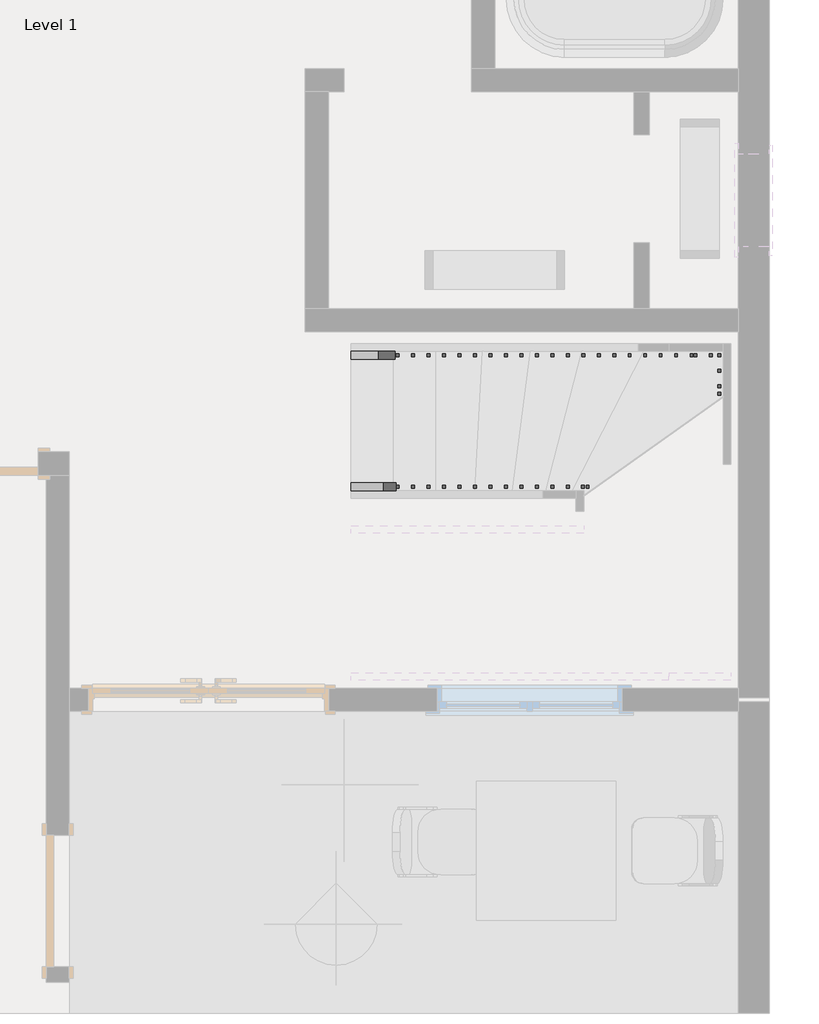
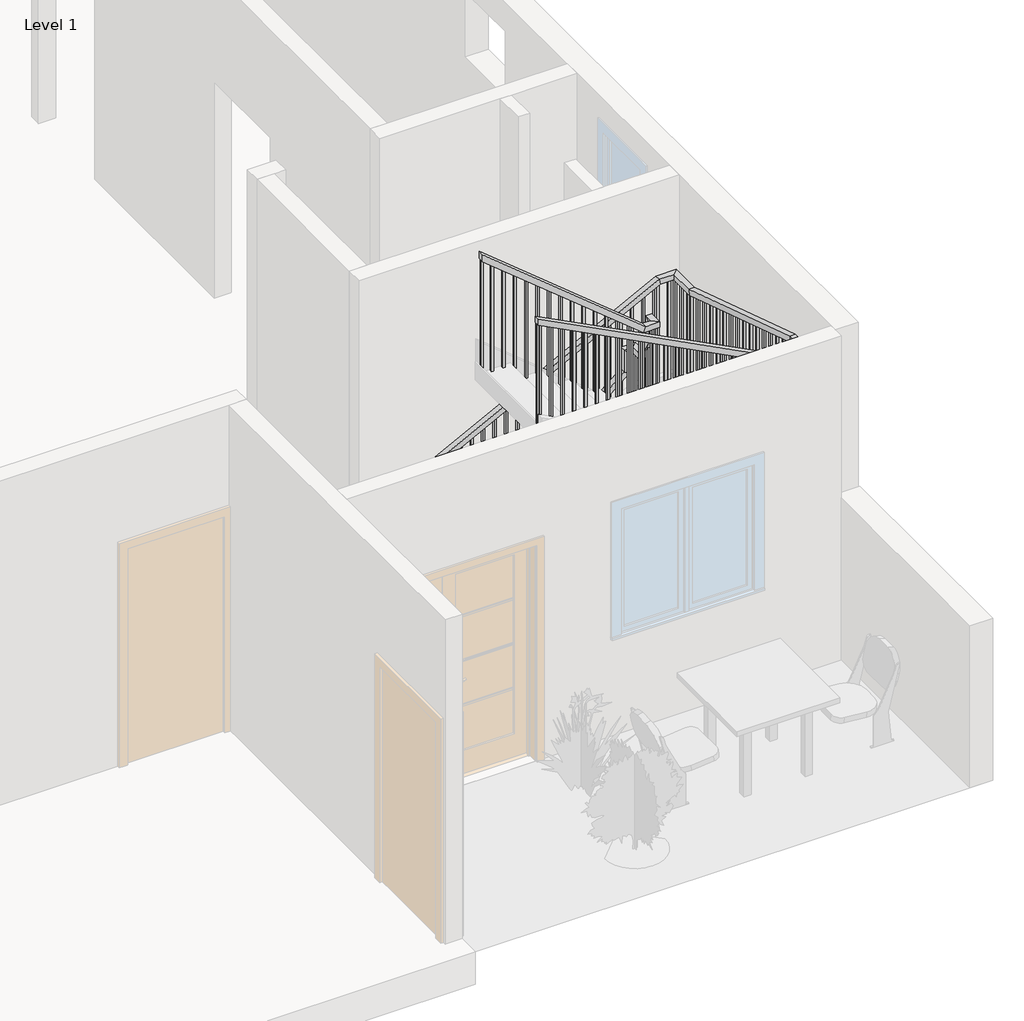
# One storey, part 2 of 3: 2 railings.
"""IFC4 building model written with IfcOpenShell, lengths in millimetres."""

from ifc_helpers import new_model, si_unit, frame, origin, place, context, project, spatial, polyline, outline, extrude, faceted_brep, element, save

model = new_model("IFC4")

# Units and contexts
model_context = context("Model", 3, world=origin())
ifc_project = project(units=[si_unit("LENGTHUNIT", "METRE", prefix="MILLI")], contexts=[model_context])

# Site, building, storey
site = spatial("IfcSite", under=ifc_project)
building = spatial("IfcBuilding", under=site)
storey = spatial("IfcBuildingStorey", under=building, Name="Level 1", Elevation=0.0)

# Railings
placement = place(None, origin())
element("IfcRailing", 1, ObjectType="Handrail - Rectangular", at=placement, inside=storey, context=model_context, shape_type="SolidModel", body=[
    faceted_brep([(-5644.7377406, -3148.8567046, 1025.2529681), (-5644.7377406, -3148.8567046, 959.7067088), (-5644.7377406, -3199.6567046, 959.7067088), (-5644.7377406, -3199.6567046, 1025.2529681), (-4193.2060487, -3148.8567046, 2208.7848338), (-4142.4060487, -3148.8567046, 2184.659247), (-4142.4060487, -3199.6567046, 2184.659247), (-4193.2060487, -3199.6567046, 2208.7848338), (-4193.2060487, -3148.8567046, 2414.6281882), (-4142.4060487, -3148.8567046, 2363.8281882), (-4142.4060487, -3199.6567046, 2363.8281882), (-4193.2060487, -3199.6567046, 2414.6281882), (-4066.2060487, -3148.8567046, 2414.6281882), (-4066.2060487, -3148.8567046, 2363.8281882), (-4117.0060487, -3199.6567046, 2363.8281882), (-4117.0060487, -3199.6567046, 2414.6281882), (-4066.2060487, -3275.8567046, 2414.6281882), (-4066.2060487, -3304.9780384, 2363.8281882), (-4117.0060487, -3304.9780384, 2363.8281882), (-4117.0060487, -3275.8567046, 2414.6281882), (-4066.2060487, -3402.8567046, 2631.5051451), (-4066.2060487, -3453.6567046, 2617.7256424), (-4117.0060487, -3453.6567046, 2617.7256424), (-4117.0060487, -3402.8567046, 2631.5051451), (-4066.2060487, -3402.8567046, 2837.3484995), (-4066.2060487, -3453.6567046, 2786.5484995), (-4117.0060487, -3453.6567046, 2786.5484995), (-4117.0060487, -3402.8567046, 2837.3484995), (-4066.2060487, -3529.8567046, 2837.3484995), (-4066.2060487, -3529.8567046, 2786.5484995), (-4117.0060487, -3479.0567046, 2786.5484995), (-4117.0060487, -3479.0567046, 2837.3484995), (-4193.2060487, -3529.8567046, 2837.3484995), (-4211.2914618, -3529.8567046, 2786.5484995), (-4211.2914618, -3479.0567046, 2786.5484995), (-4193.2060487, -3479.0567046, 2837.3484995), (-5644.7377406, -3529.8567046, 4020.8803652), (-5644.7377406, -3479.0567046, 4020.8803652), (-5644.7377406, -3479.0567046, 3955.3341059), (-5644.7377406, -3529.8567046, 3955.3341059)], [[[0, 1, 2, 3]], [[1, 0, 4, 5]], [[2, 1, 5, 6]], [[3, 2, 6, 7]], [[0, 3, 7, 4]], [[5, 4, 8, 9]], [[6, 5, 9, 10]], [[7, 6, 10, 11]], [[4, 7, 11, 8]], [[9, 8, 12, 13]], [[10, 9, 13, 14]], [[11, 10, 14, 15]], [[8, 11, 15, 12]], [[13, 12, 16, 17]], [[14, 13, 17, 18]], [[15, 14, 18, 19]], [[12, 15, 19, 16]], [[17, 16, 20, 21]], [[18, 17, 21, 22]], [[19, 18, 22, 23]], [[16, 19, 23, 20]], [[21, 20, 24, 25]], [[22, 21, 25, 26]], [[23, 22, 26, 27]], [[20, 23, 27, 24]], [[25, 24, 28, 29]], [[26, 25, 29, 30]], [[27, 26, 30, 31]], [[24, 27, 31, 28]], [[29, 28, 32, 33]], [[30, 29, 33, 34]], [[31, 30, 34, 35]], [[28, 31, 35, 32]], [[36, 37, 38, 39]], [[33, 32, 36, 39]], [[34, 33, 39, 38]], [[35, 34, 38, 37]], [[32, 35, 37, 36]]]),
    extrude(outline(polyline([(3866.2231262, -5535.4484051), (3881.7558784, -5554.4984051), (2878.6666667, -5554.4984051), (2878.6666667, -5535.4484051), (3866.2231262, -5535.4484051)])), frame((0.0, -3513.9817046, 0.0), z_axis=(0.0, 1.0, 0.0), x_axis=(0.0, 0.0, 1.0)), (0.0, 0.0, 1.0), 19.05),
    extrude(outline(polyline([(3783.3817813, -5433.8484051), (3798.9145334, -5452.8984051), (2878.6666667, -5452.8984051), (2878.6666667, -5433.8484051), (3783.3817813, -5433.8484051)])), frame((0.0, -3513.9817046, 0.0), z_axis=(0.0, 1.0, 0.0), x_axis=(0.0, 0.0, 1.0)), (0.0, 0.0, 1.0), 19.05),
    extrude(outline(polyline([(3700.5404364, -5332.2484051), (3716.0731885, -5351.2984051), (2709.3333333, -5351.2984051), (2709.3333333, -5332.2484051), (3700.5404364, -5332.2484051)])), frame((0.0, -3513.9817046, 0.0), z_axis=(0.0, 1.0, 0.0), x_axis=(0.0, 0.0, 1.0)), (0.0, 0.0, 1.0), 19.05),
    extrude(outline(polyline([(3617.6990914, -5230.6484051), (3633.2318436, -5249.6984051), (2709.3333333, -5249.6984051), (2709.3333333, -5230.6484051), (3617.6990914, -5230.6484051)])), frame((0.0, -3513.9817046, 0.0), z_axis=(0.0, 1.0, 0.0), x_axis=(0.0, 0.0, 1.0)), (0.0, 0.0, 1.0), 19.05),
    extrude(outline(polyline([(3534.8577465, -5129.0484051), (3550.3904987, -5148.0984051), (2709.3333333, -5148.0984051), (2709.3333333, -5129.0484051), (3534.8577465, -5129.0484051)])), frame((0.0, -3513.9817046, 0.0), z_axis=(0.0, 1.0, 0.0), x_axis=(0.0, 0.0, 1.0)), (0.0, 0.0, 1.0), 19.05),
    extrude(outline(polyline([(3452.0164016, -5027.4484051), (3467.5491538, -5046.4984051), (2540.0, -5046.4984051), (2540.0, -5027.4484051), (3452.0164016, -5027.4484051)])), frame((0.0, -3513.9817046, 0.0), z_axis=(0.0, 1.0, 0.0), x_axis=(0.0, 0.0, 1.0)), (0.0, 0.0, 1.0), 19.05),
    extrude(outline(polyline([(3369.1750567, -4925.8484051), (3384.7078088, -4944.8984051), (2540.0, -4944.8984051), (2540.0, -4925.8484051), (3369.1750567, -4925.8484051)])), frame((0.0, -3513.9817046, 0.0), z_axis=(0.0, 1.0, 0.0), x_axis=(0.0, 0.0, 1.0)), (0.0, 0.0, 1.0), 19.05),
    extrude(outline(polyline([(3286.3337117, -4824.2484051), (3301.8664639, -4843.2984051), (2540.0, -4843.2984051), (2540.0, -4824.2484051), (3286.3337117, -4824.2484051)])), frame((0.0, -3513.9817046, 0.0), z_axis=(0.0, 1.0, 0.0), x_axis=(0.0, 0.0, 1.0)), (0.0, 0.0, 1.0), 19.05),
    extrude(outline(polyline([(3203.4923668, -4722.6484051), (3219.025119, -4741.6984051), (2370.6666667, -4741.6984051), (2370.6666667, -4722.6484051), (3203.4923668, -4722.6484051)])), frame((0.0, -3513.9817046, 0.0), z_axis=(0.0, 1.0, 0.0), x_axis=(0.0, 0.0, 1.0)), (0.0, 0.0, 1.0), 19.05),
    extrude(outline(polyline([(3120.6510219, -4621.0484051), (3136.1837741, -4640.0984051), (2370.6666667, -4640.0984051), (2370.6666667, -4621.0484051), (3120.6510219, -4621.0484051)])), frame((0.0, -3513.9817046, 0.0), z_axis=(0.0, 1.0, 0.0), x_axis=(0.0, 0.0, 1.0)), (0.0, 0.0, 1.0), 19.05),
    extrude(outline(polyline([(3037.809677, -4519.4484051), (3053.3424291, -4538.4984051), (2201.3333333, -4538.4984051), (2201.3333333, -4519.4484051), (3037.809677, -4519.4484051)])), frame((0.0, -3513.9817046, 0.0), z_axis=(0.0, 1.0, 0.0), x_axis=(0.0, 0.0, 1.0)), (0.0, 0.0, 1.0), 19.05),
    extrude(outline(polyline([(2954.9683321, -4417.8484051), (2970.5010842, -4436.8984051), (2201.3333333, -4436.8984051), (2201.3333333, -4417.8484051), (2954.9683321, -4417.8484051)])), frame((0.0, -3513.9817046, 0.0), z_axis=(0.0, 1.0, 0.0), x_axis=(0.0, 0.0, 1.0)), (0.0, 0.0, 1.0), 19.05),
    extrude(outline(polyline([(2872.1269871, -4316.2484051), (2887.6597393, -4335.2984051), (2032.0, -4335.2984051), (2032.0, -4316.2484051), (2872.1269871, -4316.2484051)])), frame((0.0, -3513.9817046, 0.0), z_axis=(0.0, 1.0, 0.0), x_axis=(0.0, 0.0, 1.0)), (0.0, 0.0, 1.0), 19.05),
    extrude(outline(polyline([(2789.2856422, -4214.6484051), (2804.8183944, -4233.6984051), (2032.0, -4233.6984051), (2032.0, -4214.6484051), (2789.2856422, -4214.6484051)])), frame((0.0, -3513.9817046, 0.0), z_axis=(0.0, 1.0, 0.0), x_axis=(0.0, 0.0, 1.0)), (0.0, 0.0, 1.0), 19.05),
    extrude(outline(polyline([(-3401.7676083, 2529.115018), (-3382.7176083, 2496.5834745), (-3382.7176083, 1524.0), (-3401.7676083, 1524.0), (-3401.7676083, 2529.115018)])), frame((-4101.1310487, 0.0, 0.0), z_axis=(1.0, 0.0, 0.0), x_axis=(0.0, 1.0, 0.0)), (0.0, 0.0, 1.0), 19.05),
    extrude(outline(polyline([(-3300.1676083, 2355.6134525), (-3281.1176083, 2323.0819089), (-3281.1176083, 1524.0), (-3300.1676083, 1524.0), (-3300.1676083, 2355.6134525)])), frame((-4101.1310487, 0.0, 0.0), z_axis=(1.0, 0.0, 0.0), x_axis=(0.0, 1.0, 0.0)), (0.0, 0.0, 1.0), 19.05),
    extrude(outline(polyline([(2127.2519138, -4212.8127406), (2111.7191617, -4231.8627406), (1016.0, -4231.8627406), (1016.0, -4212.8127406), (2127.2519138, -4212.8127406)])), frame((0.0, -3183.7817046, 0.0), z_axis=(0.0, 1.0, 0.0), x_axis=(0.0, 0.0, 1.0)), (0.0, 0.0, 1.0), 19.05),
    extrude(outline(polyline([(2044.4105689, -4314.4127406), (2028.8778167, -4333.4627406), (1016.0, -4333.4627406), (1016.0, -4314.4127406), (2044.4105689, -4314.4127406)])), frame((0.0, -3183.7817046, 0.0), z_axis=(0.0, 1.0, 0.0), x_axis=(0.0, 0.0, 1.0)), (0.0, 0.0, 1.0), 19.05),
    extrude(outline(polyline([(1961.569224, -4416.0127406), (1946.0364718, -4435.0627406), (846.6666667, -4435.0627406), (846.6666667, -4416.0127406), (1961.569224, -4416.0127406)])), frame((0.0, -3183.7817046, 0.0), z_axis=(0.0, 1.0, 0.0), x_axis=(0.0, 0.0, 1.0)), (0.0, 0.0, 1.0), 19.05),
    extrude(outline(polyline([(1878.7278791, -4517.6127406), (1863.1951269, -4536.6627406), (846.6666667, -4536.6627406), (846.6666667, -4517.6127406), (1878.7278791, -4517.6127406)])), frame((0.0, -3183.7817046, 0.0), z_axis=(0.0, 1.0, 0.0), x_axis=(0.0, 0.0, 1.0)), (0.0, 0.0, 1.0), 19.05),
    extrude(outline(polyline([(1795.8865341, -4619.2127406), (1780.353782, -4638.2627406), (677.3333333, -4638.2627406), (677.3333333, -4619.2127406), (1795.8865341, -4619.2127406)])), frame((0.0, -3183.7817046, 0.0), z_axis=(0.0, 1.0, 0.0), x_axis=(0.0, 0.0, 1.0)), (0.0, 0.0, 1.0), 19.05),
    extrude(outline(polyline([(1713.0451892, -4720.8127406), (1697.5124371, -4739.8627406), (677.3333333, -4739.8627406), (677.3333333, -4720.8127406), (1713.0451892, -4720.8127406)])), frame((0.0, -3183.7817046, 0.0), z_axis=(0.0, 1.0, 0.0), x_axis=(0.0, 0.0, 1.0)), (0.0, 0.0, 1.0), 19.05),
    extrude(outline(polyline([(1630.2038443, -4822.4127406), (1614.6710921, -4841.4627406), (508.0, -4841.4627406), (508.0, -4822.4127406), (1630.2038443, -4822.4127406)])), frame((0.0, -3183.7817046, 0.0), z_axis=(0.0, 1.0, 0.0), x_axis=(0.0, 0.0, 1.0)), (0.0, 0.0, 1.0), 19.05),
    extrude(outline(polyline([(1547.3624994, -4924.0127406), (1531.8297472, -4943.0627406), (508.0, -4943.0627406), (508.0, -4924.0127406), (1547.3624994, -4924.0127406)])), frame((0.0, -3183.7817046, 0.0), z_axis=(0.0, 1.0, 0.0), x_axis=(0.0, 0.0, 1.0)), (0.0, 0.0, 1.0), 19.05),
    extrude(outline(polyline([(1464.5211545, -5025.6127406), (1448.9884023, -5044.6627406), (508.0, -5044.6627406), (508.0, -5025.6127406), (1464.5211545, -5025.6127406)])), frame((0.0, -3183.7817046, 0.0), z_axis=(0.0, 1.0, 0.0), x_axis=(0.0, 0.0, 1.0)), (0.0, 0.0, 1.0), 19.05),
    extrude(outline(polyline([(1381.6798095, -5127.2127406), (1366.1470574, -5146.2627406), (338.6666667, -5146.2627406), (338.6666667, -5127.2127406), (1381.6798095, -5127.2127406)])), frame((0.0, -3183.7817046, 0.0), z_axis=(0.0, 1.0, 0.0), x_axis=(0.0, 0.0, 1.0)), (0.0, 0.0, 1.0), 19.05),
    extrude(outline(polyline([(1298.8384646, -5228.8127406), (1283.3057124, -5247.8627406), (338.6666667, -5247.8627406), (338.6666667, -5228.8127406), (1298.8384646, -5228.8127406)])), frame((0.0, -3183.7817046, 0.0), z_axis=(0.0, 1.0, 0.0), x_axis=(0.0, 0.0, 1.0)), (0.0, 0.0, 1.0), 19.05),
    extrude(outline(polyline([(1215.9971197, -5330.4127406), (1200.4643675, -5349.4627406), (338.6666667, -5349.4627406), (338.6666667, -5330.4127406), (1215.9971197, -5330.4127406)])), frame((0.0, -3183.7817046, 0.0), z_axis=(0.0, 1.0, 0.0), x_axis=(0.0, 0.0, 1.0)), (0.0, 0.0, 1.0), 19.05),
    extrude(outline(polyline([(1133.1557748, -5432.0127406), (1117.6230226, -5451.0627406), (169.3333333, -5451.0627406), (169.3333333, -5432.0127406), (1133.1557748, -5432.0127406)])), frame((0.0, -3183.7817046, 0.0), z_axis=(0.0, 1.0, 0.0), x_axis=(0.0, 0.0, 1.0)), (0.0, 0.0, 1.0), 19.05),
    extrude(outline(polyline([(1050.3144298, -5533.6127406), (1034.7816777, -5552.6627406), (169.3333333, -5552.6627406), (169.3333333, -5533.6127406), (1050.3144298, -5533.6127406)])), frame((0.0, -3183.7817046, 0.0), z_axis=(0.0, 1.0, 0.0), x_axis=(0.0, 0.0, 1.0)), (0.0, 0.0, 1.0), 19.05),
    extrude(outline(polyline([(-4113.0484051, -3494.9317046), (-4113.0484051, -3513.9817046), (-4132.0984051, -3513.9817046), (-4132.0984051, -3494.9317046), (-4113.0484051, -3494.9317046)])), frame((0.0, 0.0, 1862.6666667), z_axis=(0.0, 0.0, 1.0), x_axis=(1.0, 0.0, 0.0)), (0.0, 0.0, 1.0), 923.8818329),
    extrude(outline(polyline([(-4101.1310487, -3494.9317046), (-4082.0810487, -3494.9317046), (-4082.0810487, -3513.9817046), (-4101.1310487, -3513.9817046), (-4101.1310487, -3494.9317046)])), frame((0.0, 0.0, 1862.6666667), z_axis=(0.0, 0.0, 1.0), x_axis=(1.0, 0.0, 0.0)), (0.0, 0.0, 1.0), 923.8818329),
    extrude(outline(polyline([(-4101.1310487, -3480.1458008), (-4082.0810487, -3480.1458008), (-4082.0810487, -3499.1958008), (-4101.1310487, -3499.1958008), (-4101.1310487, -3480.1458008)])), frame((0.0, 0.0, 1693.3333333), z_axis=(0.0, 0.0, 1.0), x_axis=(1.0, 0.0, 0.0)), (0.0, 0.0, 1.0), 1093.2151662),
    extrude(outline(polyline([(-4101.1310487, -3179.5176083), (-4082.0810487, -3179.5176083), (-4082.0810487, -3198.5676083), (-4101.1310487, -3198.5676083), (-4101.1310487, -3179.5176083)])), frame((0.0, 0.0, 1354.6666667), z_axis=(0.0, 0.0, 1.0), x_axis=(1.0, 0.0, 0.0)), (0.0, 0.0, 1.0), 1009.1615215),
    extrude(outline(polyline([(-4101.1310487, -3183.7817046), (-4101.1310487, -3164.7317046), (-4082.0810487, -3164.7317046), (-4082.0810487, -3183.7817046), (-4101.1310487, -3183.7817046)])), frame((0.0, 0.0, 1185.3333333), z_axis=(0.0, 0.0, 1.0), x_axis=(1.0, 0.0, 0.0)), (0.0, 0.0, 1.0), 1178.4948549),
    extrude(outline(polyline([(-4132.0984051, -3183.7817046), (-4132.0984051, -3164.7317046), (-4113.0484051, -3164.7317046), (-4113.0484051, -3183.7817046), (-4132.0984051, -3183.7817046)])), frame((0.0, 0.0, 1185.3333333), z_axis=(0.0, 0.0, 1.0), x_axis=(1.0, 0.0, 0.0)), (0.0, 0.0, 1.0), 1178.4948549),
    extrude(outline(polyline([(3939.8013537, -5625.6877406), (3955.3341059, -5644.7377406), (2878.6666667, -5644.7377406), (2878.6666667, -5625.6877406), (3939.8013537, -5625.6877406)])), frame((0.0, -3513.9817046, 0.0), z_axis=(0.0, 1.0, 0.0), x_axis=(0.0, 0.0, 1.0)), (0.0, 0.0, 1.0), 19.05),
    extrude(outline(polyline([(975.239461, -5625.6877406), (959.7067088, -5644.7377406), (169.3333333, -5644.7377406), (169.3333333, -5625.6877406), (975.239461, -5625.6877406)])), frame((0.0, -3183.7817046, 0.0), z_axis=(0.0, 1.0, 0.0), x_axis=(0.0, 0.0, 1.0)), (0.0, 0.0, 1.0), 19.05),
])
element("IfcRailing", 2, ObjectType="Handrail - Rectangular", at=placement, inside=storey, context=model_context, shape_type="SolidModel", body=[
    faceted_brep([(-5644.7377406, -2285.2567046, 1109.0771751), (-5644.7377406, -2285.2567046, 1051.9280057), (-5644.7377406, -2336.0567046, 1051.9280057), (-5644.7377406, -2336.0567046, 1109.0771751), (-3384.7558841, -2285.2567046, 2273.7644996), (-3372.4358328, -2285.2567046, 2222.9644996), (-3372.4358328, -2336.0567046, 2222.9644996), (-3384.7558841, -2336.0567046, 2273.7644996), (-3202.6060487, -2285.2567046, 2273.7644996), (-3202.6060487, -2285.2567046, 2222.9644996), (-3253.4060487, -2336.0567046, 2222.9644996), (-3253.4060487, -2336.0567046, 2273.7644996), (-3202.6060487, -2562.4106572, 2273.7644996), (-3202.6060487, -2570.3612333, 2222.9644996), (-3253.4060487, -2570.3612333, 2222.9644996), (-3253.4060487, -2562.4106572, 2273.7644996), (-3202.6060487, -4116.3027519, 2772.3688337), (-3202.6060487, -4124.2533281, 2721.5688337), (-3253.4060487, -4124.2533281, 2721.5688337), (-3253.4060487, -4116.3027519, 2772.3688337), (-3202.6060487, -4393.4567046, 2772.3688337), (-3202.6060487, -4393.4567046, 2721.5688337), (-3253.4060487, -4342.6567046, 2721.5688337), (-3253.4060487, -4342.6567046, 2772.3688337), (-3384.7558841, -4393.4567046, 2772.3688337), (-3397.0759354, -4393.4567046, 2721.5688337), (-3397.0759354, -4342.6567046, 2721.5688337), (-3384.7558841, -4342.6567046, 2772.3688337), (-5644.7377406, -4393.4567046, 3937.0561582), (-5644.7377406, -4342.6567046, 3937.0561582), (-5644.7377406, -4342.6567046, 3879.9069889), (-5644.7377406, -4393.4567046, 3879.9069889)], [[[0, 1, 2, 3]], [[1, 0, 4, 5]], [[2, 1, 5, 6]], [[3, 2, 6, 7]], [[0, 3, 7, 4]], [[5, 4, 8, 9]], [[6, 5, 9, 10]], [[7, 6, 10, 11]], [[4, 7, 11, 8]], [[9, 8, 12, 13]], [[10, 9, 13, 14]], [[11, 10, 14, 15]], [[8, 11, 15, 12]], [[13, 12, 16, 17]], [[14, 13, 17, 18]], [[15, 14, 18, 19]], [[12, 15, 19, 16]], [[17, 16, 20, 21]], [[18, 17, 21, 22]], [[19, 18, 22, 23]], [[16, 19, 23, 20]], [[21, 20, 24, 25]], [[22, 21, 25, 26]], [[23, 22, 26, 27]], [[20, 23, 27, 24]], [[28, 29, 30, 31]], [[25, 24, 28, 31]], [[26, 25, 31, 30]], [[27, 26, 30, 29]], [[24, 27, 29, 28]]]),
    extrude(outline(polyline([(3872.0443296, -5629.4808841), (2878.6666667, -5629.4808841), (2878.6666667, -5610.4308841), (3862.2268642, -5610.4308841), (3872.0443296, -5629.4808841)])), frame((0.0, -4377.5817046, 0.0), z_axis=(0.0, 1.0, 0.0), x_axis=(0.0, 0.0, 1.0)), (0.0, 0.0, 1.0), 19.05),
    extrude(outline(polyline([(3819.6845145, -5527.8808841), (2878.6666667, -5527.8808841), (2878.6666667, -5508.8308841), (3809.8670491, -5508.8308841), (3819.6845145, -5527.8808841)])), frame((0.0, -4377.5817046, 0.0), z_axis=(0.0, 1.0, 0.0), x_axis=(0.0, 0.0, 1.0)), (0.0, 0.0, 1.0), 19.05),
    extrude(outline(polyline([(3767.3246993, -5426.2808841), (2878.6666667, -5426.2808841), (2878.6666667, -5407.2308841), (3757.507234, -5407.2308841), (3767.3246993, -5426.2808841)])), frame((0.0, -4377.5817046, 0.0), z_axis=(0.0, 1.0, 0.0), x_axis=(0.0, 0.0, 1.0)), (0.0, 0.0, 1.0), 19.05),
    extrude(outline(polyline([(3714.9648842, -5324.6808841), (2709.3333333, -5324.6808841), (2709.3333333, -5305.6308841), (3705.1474189, -5305.6308841), (3714.9648842, -5324.6808841)])), frame((0.0, -4377.5817046, 0.0), z_axis=(0.0, 1.0, 0.0), x_axis=(0.0, 0.0, 1.0)), (0.0, 0.0, 1.0), 19.05),
    extrude(outline(polyline([(3662.6050691, -5223.0808841), (2709.3333333, -5223.0808841), (2709.3333333, -5204.0308841), (3652.7876038, -5204.0308841), (3662.6050691, -5223.0808841)])), frame((0.0, -4377.5817046, 0.0), z_axis=(0.0, 1.0, 0.0), x_axis=(0.0, 0.0, 1.0)), (0.0, 0.0, 1.0), 19.05),
    extrude(outline(polyline([(3610.245254, -5121.4808841), (2709.3333333, -5121.4808841), (2709.3333333, -5102.4308841), (3600.4277887, -5102.4308841), (3610.245254, -5121.4808841)])), frame((0.0, -4377.5817046, 0.0), z_axis=(0.0, 1.0, 0.0), x_axis=(0.0, 0.0, 1.0)), (0.0, 0.0, 1.0), 19.05),
    extrude(outline(polyline([(3557.8854389, -5019.8808841), (2540.0, -5019.8808841), (2540.0, -5000.8308841), (3548.0679735, -5000.8308841), (3557.8854389, -5019.8808841)])), frame((0.0, -4377.5817046, 0.0), z_axis=(0.0, 1.0, 0.0), x_axis=(0.0, 0.0, 1.0)), (0.0, 0.0, 1.0), 19.05),
    extrude(outline(polyline([(3505.5256238, -4918.2808841), (2540.0, -4918.2808841), (2540.0, -4899.2308841), (3495.7081584, -4899.2308841), (3505.5256238, -4918.2808841)])), frame((0.0, -4377.5817046, 0.0), z_axis=(0.0, 1.0, 0.0), x_axis=(0.0, 0.0, 1.0)), (0.0, 0.0, 1.0), 19.05),
    extrude(outline(polyline([(3453.1658086, -4816.6808841), (2540.0, -4816.6808841), (2540.0, -4797.6308841), (3443.3483433, -4797.6308841), (3453.1658086, -4816.6808841)])), frame((0.0, -4377.5817046, 0.0), z_axis=(0.0, 1.0, 0.0), x_axis=(0.0, 0.0, 1.0)), (0.0, 0.0, 1.0), 19.05),
    extrude(outline(polyline([(3400.8059935, -4715.0808841), (2370.6666667, -4715.0808841), (2370.6666667, -4696.0308841), (3390.9885282, -4696.0308841), (3400.8059935, -4715.0808841)])), frame((0.0, -4377.5817046, 0.0), z_axis=(0.0, 1.0, 0.0), x_axis=(0.0, 0.0, 1.0)), (0.0, 0.0, 1.0), 19.05),
    extrude(outline(polyline([(3348.4461784, -4613.4808841), (2370.6666667, -4613.4808841), (2370.6666667, -4594.4308841), (3338.6287131, -4594.4308841), (3348.4461784, -4613.4808841)])), frame((0.0, -4377.5817046, 0.0), z_axis=(0.0, 1.0, 0.0), x_axis=(0.0, 0.0, 1.0)), (0.0, 0.0, 1.0), 19.05),
    extrude(outline(polyline([(3296.0863633, -4511.8808841), (2370.6666667, -4511.8808841), (2370.6666667, -4492.8308841), (3286.268898, -4492.8308841), (3296.0863633, -4511.8808841)])), frame((0.0, -4377.5817046, 0.0), z_axis=(0.0, 1.0, 0.0), x_axis=(0.0, 0.0, 1.0)), (0.0, 0.0, 1.0), 19.05),
    extrude(outline(polyline([(3243.7265482, -4410.2808841), (2201.3333333, -4410.2808841), (2201.3333333, -4391.2308841), (3233.9090828, -4391.2308841), (3243.7265482, -4410.2808841)])), frame((0.0, -4377.5817046, 0.0), z_axis=(0.0, 1.0, 0.0), x_axis=(0.0, 0.0, 1.0)), (0.0, 0.0, 1.0), 19.05),
    extrude(outline(polyline([(3191.3667331, -4308.6808841), (2201.3333333, -4308.6808841), (2201.3333333, -4289.6308841), (3181.5492677, -4289.6308841), (3191.3667331, -4308.6808841)])), frame((0.0, -4377.5817046, 0.0), z_axis=(0.0, 1.0, 0.0), x_axis=(0.0, 0.0, 1.0)), (0.0, 0.0, 1.0), 19.05),
    extrude(outline(polyline([(3139.0069179, -4207.0808841), (2201.3333333, -4207.0808841), (2201.3333333, -4188.0308841), (3129.1894526, -4188.0308841), (3139.0069179, -4207.0808841)])), frame((0.0, -4377.5817046, 0.0), z_axis=(0.0, 1.0, 0.0), x_axis=(0.0, 0.0, 1.0)), (0.0, 0.0, 1.0), 19.05),
    extrude(outline(polyline([(3086.6471028, -4105.4808841), (2032.0, -4105.4808841), (2032.0, -4086.4308841), (3076.8296375, -4086.4308841), (3086.6471028, -4105.4808841)])), frame((0.0, -4377.5817046, 0.0), z_axis=(0.0, 1.0, 0.0), x_axis=(0.0, 0.0, 1.0)), (0.0, 0.0, 1.0), 19.05),
    extrude(outline(polyline([(3034.2872877, -4003.8808841), (2032.0, -4003.8808841), (2032.0, -3984.8308841), (3024.4698224, -3984.8308841), (3034.2872877, -4003.8808841)])), frame((0.0, -4377.5817046, 0.0), z_axis=(0.0, 1.0, 0.0), x_axis=(0.0, 0.0, 1.0)), (0.0, 0.0, 1.0), 19.05),
    extrude(outline(polyline([(2981.9274726, -3902.2808841), (2032.0, -3902.2808841), (2032.0, -3883.2308841), (2972.1100073, -3883.2308841), (2981.9274726, -3902.2808841)])), frame((0.0, -4377.5817046, 0.0), z_axis=(0.0, 1.0, 0.0), x_axis=(0.0, 0.0, 1.0)), (0.0, 0.0, 1.0), 19.05),
    extrude(outline(polyline([(2929.5676575, -3800.6808841), (2032.0, -3800.6808841), (2032.0, -3781.6308841), (2919.7501921, -3781.6308841), (2929.5676575, -3800.6808841)])), frame((0.0, -4377.5817046, 0.0), z_axis=(0.0, 1.0, 0.0), x_axis=(0.0, 0.0, 1.0)), (0.0, 0.0, 1.0), 19.05),
    extrude(outline(polyline([(2877.2078424, -3699.0808841), (1862.6666667, -3699.0808841), (1862.6666667, -3680.0308841), (2867.390377, -3680.0308841), (2877.2078424, -3699.0808841)])), frame((0.0, -4377.5817046, 0.0), z_axis=(0.0, 1.0, 0.0), x_axis=(0.0, 0.0, 1.0)), (0.0, 0.0, 1.0), 19.05),
    extrude(outline(polyline([(2824.8480272, -3597.4808841), (1862.6666667, -3597.4808841), (1862.6666667, -3578.4308841), (2815.0305619, -3578.4308841), (2824.8480272, -3597.4808841)])), frame((0.0, -4377.5817046, 0.0), z_axis=(0.0, 1.0, 0.0), x_axis=(0.0, 0.0, 1.0)), (0.0, 0.0, 1.0), 19.05),
    extrude(outline(polyline([(2772.4882121, -3495.8808841), (1862.6666667, -3495.8808841), (1862.6666667, -3476.8308841), (2762.6707468, -3476.8308841), (2772.4882121, -3495.8808841)])), frame((0.0, -4377.5817046, 0.0), z_axis=(0.0, 1.0, 0.0), x_axis=(0.0, 0.0, 1.0)), (0.0, 0.0, 1.0), 19.05),
    extrude(outline(polyline([(-3320.0810487, -4377.5817046), (-3339.1310487, -4377.5817046), (-3339.1310487, -4358.5317046), (-3320.0810487, -4358.5317046), (-3320.0810487, -4377.5817046)])), frame((0.0, 0.0, 1862.6666667), z_axis=(0.0, 0.0, 1.0), x_axis=(1.0, 0.0, 0.0)), (0.0, 0.0, 1.0), 858.902167),
    extrude(outline(polyline([(-3218.4810487, -4309.9777519), (-3218.4810487, -4329.0277519), (-3237.5310487, -4329.0277519), (-3237.5310487, -4309.9777519), (-3218.4810487, -4309.9777519)])), frame((0.0, 0.0, 1862.6666667), z_axis=(0.0, 0.0, 1.0), x_axis=(1.0, 0.0, 0.0)), (0.0, 0.0, 1.0), 858.902167),
    extrude(outline(polyline([(-3218.4810487, -4208.3777519), (-3218.4810487, -4227.4277519), (-3237.5310487, -4227.4277519), (-3237.5310487, -4208.3777519), (-3218.4810487, -4208.3777519)])), frame((0.0, 0.0, 1862.6666667), z_axis=(0.0, 0.0, 1.0), x_axis=(1.0, 0.0, 0.0)), (0.0, 0.0, 1.0), 858.902167),
    extrude(outline(polyline([(-4076.8856572, 2706.3697564), (-4076.8856572, 1693.3333333), (-4095.9356572, 1693.3333333), (-4095.9356572, 2712.4824155), (-4076.8856572, 2706.3697564)])), frame((-3237.5310487, 0.0, 0.0), z_axis=(1.0, 0.0, 0.0), x_axis=(0.0, 1.0, 0.0)), (0.0, 0.0, 1.0), 19.05),
    extrude(outline(polyline([(-3975.2856572, 2673.7689082), (-3975.2856572, 1693.3333333), (-3994.3356572, 1693.3333333), (-3994.3356572, 2679.8815673), (-3975.2856572, 2673.7689082)])), frame((-3237.5310487, 0.0, 0.0), z_axis=(1.0, 0.0, 0.0), x_axis=(0.0, 1.0, 0.0)), (0.0, 0.0, 1.0), 19.05),
    extrude(outline(polyline([(-3873.6856572, 2641.16806), (-3873.6856572, 1693.3333333), (-3892.7356572, 1693.3333333), (-3892.7356572, 2647.280719), (-3873.6856572, 2641.16806)])), frame((-3237.5310487, 0.0, 0.0), z_axis=(1.0, 0.0, 0.0), x_axis=(0.0, 1.0, 0.0)), (0.0, 0.0, 1.0), 19.05),
    extrude(outline(polyline([(-3772.0856572, 2608.5672118), (-3772.0856572, 1693.3333333), (-3791.1356572, 1693.3333333), (-3791.1356572, 2614.6798708), (-3772.0856572, 2608.5672118)])), frame((-3237.5310487, 0.0, 0.0), z_axis=(1.0, 0.0, 0.0), x_axis=(0.0, 1.0, 0.0)), (0.0, 0.0, 1.0), 19.05),
    extrude(outline(polyline([(-3670.4856572, 2575.9663635), (-3670.4856572, 1693.3333333), (-3689.5356572, 1693.3333333), (-3689.5356572, 2582.0790226), (-3670.4856572, 2575.9663635)])), frame((-3237.5310487, 0.0, 0.0), z_axis=(1.0, 0.0, 0.0), x_axis=(0.0, 1.0, 0.0)), (0.0, 0.0, 1.0), 19.05),
    extrude(outline(polyline([(-3568.8856572, 2543.3655153), (-3568.8856572, 1693.3333333), (-3587.9356572, 1693.3333333), (-3587.9356572, 2549.4781744), (-3568.8856572, 2543.3655153)])), frame((-3237.5310487, 0.0, 0.0), z_axis=(1.0, 0.0, 0.0), x_axis=(0.0, 1.0, 0.0)), (0.0, 0.0, 1.0), 19.05),
    extrude(outline(polyline([(-3467.2856572, 2510.7646671), (-3467.2856572, 1524.0), (-3486.3356572, 1524.0), (-3486.3356572, 2516.8773261), (-3467.2856572, 2510.7646671)])), frame((-3237.5310487, 0.0, 0.0), z_axis=(1.0, 0.0, 0.0), x_axis=(0.0, 1.0, 0.0)), (0.0, 0.0, 1.0), 19.05),
    extrude(outline(polyline([(-3365.6856572, 2478.1638189), (-3365.6856572, 1524.0), (-3384.7356572, 1524.0), (-3384.7356572, 2484.2764779), (-3365.6856572, 2478.1638189)])), frame((-3237.5310487, 0.0, 0.0), z_axis=(1.0, 0.0, 0.0), x_axis=(0.0, 1.0, 0.0)), (0.0, 0.0, 1.0), 19.05),
    extrude(outline(polyline([(-3264.0856572, 2445.5629706), (-3264.0856572, 1524.0), (-3283.1356572, 1524.0), (-3283.1356572, 2451.6756297), (-3264.0856572, 2445.5629706)])), frame((-3237.5310487, 0.0, 0.0), z_axis=(1.0, 0.0, 0.0), x_axis=(0.0, 1.0, 0.0)), (0.0, 0.0, 1.0), 19.05),
    extrude(outline(polyline([(-3162.4856572, 2412.9621224), (-3162.4856572, 1524.0), (-3181.5356572, 1524.0), (-3181.5356572, 2419.0747814), (-3162.4856572, 2412.9621224)])), frame((-3237.5310487, 0.0, 0.0), z_axis=(1.0, 0.0, 0.0), x_axis=(0.0, 1.0, 0.0)), (0.0, 0.0, 1.0), 19.05),
    extrude(outline(polyline([(-3060.8856572, 2380.3612742), (-3060.8856572, 1354.6666667), (-3079.9356572, 1354.6666667), (-3079.9356572, 2386.4739332), (-3060.8856572, 2380.3612742)])), frame((-3237.5310487, 0.0, 0.0), z_axis=(1.0, 0.0, 0.0), x_axis=(0.0, 1.0, 0.0)), (0.0, 0.0, 1.0), 19.05),
    extrude(outline(polyline([(-2959.2856572, 2347.7604259), (-2959.2856572, 1354.6666667), (-2978.3356572, 1354.6666667), (-2978.3356572, 2353.873085), (-2959.2856572, 2347.7604259)])), frame((-3237.5310487, 0.0, 0.0), z_axis=(1.0, 0.0, 0.0), x_axis=(0.0, 1.0, 0.0)), (0.0, 0.0, 1.0), 19.05),
    extrude(outline(polyline([(-2857.6856572, 2315.1595777), (-2857.6856572, 1354.6666667), (-2876.7356572, 1354.6666667), (-2876.7356572, 2321.2722368), (-2857.6856572, 2315.1595777)])), frame((-3237.5310487, 0.0, 0.0), z_axis=(1.0, 0.0, 0.0), x_axis=(0.0, 1.0, 0.0)), (0.0, 0.0, 1.0), 19.05),
    extrude(outline(polyline([(-2756.0856572, 2282.5587295), (-2756.0856572, 1354.6666667), (-2775.1356572, 1354.6666667), (-2775.1356572, 2288.6713885), (-2756.0856572, 2282.5587295)])), frame((-3237.5310487, 0.0, 0.0), z_axis=(1.0, 0.0, 0.0), x_axis=(0.0, 1.0, 0.0)), (0.0, 0.0, 1.0), 19.05),
    extrude(outline(polyline([(-2654.4856572, 2249.9578813), (-2654.4856572, 1354.6666667), (-2673.5356572, 1354.6666667), (-2673.5356572, 2256.0705403), (-2654.4856572, 2249.9578813)])), frame((-3237.5310487, 0.0, 0.0), z_axis=(1.0, 0.0, 0.0), x_axis=(0.0, 1.0, 0.0)), (0.0, 0.0, 1.0), 19.05),
    extrude(outline(polyline([(-3218.4810487, -2504.3317046), (-3218.4810487, -2523.3817046), (-3237.5310487, -2523.3817046), (-3237.5310487, -2504.3317046), (-3218.4810487, -2504.3317046)])), frame((0.0, 0.0, 1185.3333333), z_axis=(0.0, 0.0, 1.0), x_axis=(1.0, 0.0, 0.0)), (0.0, 0.0, 1.0), 1037.6311663),
    extrude(outline(polyline([(-3218.4810487, -2402.7317046), (-3218.4810487, -2421.7817046), (-3237.5310487, -2421.7817046), (-3237.5310487, -2402.7317046), (-3218.4810487, -2402.7317046)])), frame((0.0, 0.0, 1185.3333333), z_axis=(0.0, 0.0, 1.0), x_axis=(1.0, 0.0, 0.0)), (0.0, 0.0, 1.0), 1037.6311663),
    extrude(outline(polyline([(-3292.6808841, -2301.1317046), (-3273.6308841, -2301.1317046), (-3273.6308841, -2320.1817046), (-3292.6808841, -2320.1817046), (-3292.6808841, -2301.1317046)])), frame((0.0, 0.0, 1185.3333333), z_axis=(0.0, 0.0, 1.0), x_axis=(1.0, 0.0, 0.0)), (0.0, 0.0, 1.0), 1037.6311663),
    extrude(outline(polyline([(2198.9352056, -3419.0627406), (1185.3333333, -3419.0627406), (1185.3333333, -3400.0127406), (2208.752671, -3400.0127406), (2198.9352056, -3419.0627406)])), frame((0.0, -2320.1817046, 0.0), z_axis=(0.0, 1.0, 0.0), x_axis=(0.0, 0.0, 1.0)), (0.0, 0.0, 1.0), 19.05),
    extrude(outline(polyline([(2146.5753905, -3520.6627406), (1185.3333333, -3520.6627406), (1185.3333333, -3501.6127406), (2156.3928558, -3501.6127406), (2146.5753905, -3520.6627406)])), frame((0.0, -2320.1817046, 0.0), z_axis=(0.0, 1.0, 0.0), x_axis=(0.0, 0.0, 1.0)), (0.0, 0.0, 1.0), 19.05),
    extrude(outline(polyline([(2094.2155754, -3622.2627406), (1185.3333333, -3622.2627406), (1185.3333333, -3603.2127406), (2104.0330407, -3603.2127406), (2094.2155754, -3622.2627406)])), frame((0.0, -2320.1817046, 0.0), z_axis=(0.0, 1.0, 0.0), x_axis=(0.0, 0.0, 1.0)), (0.0, 0.0, 1.0), 19.05),
    extrude(outline(polyline([(2041.8557603, -3723.8627406), (1185.3333333, -3723.8627406), (1185.3333333, -3704.8127406), (2051.6732256, -3704.8127406), (2041.8557603, -3723.8627406)])), frame((0.0, -2320.1817046, 0.0), z_axis=(0.0, 1.0, 0.0), x_axis=(0.0, 0.0, 1.0)), (0.0, 0.0, 1.0), 19.05),
    extrude(outline(polyline([(1989.4959452, -3825.4627406), (1016.0, -3825.4627406), (1016.0, -3806.4127406), (1999.3134105, -3806.4127406), (1989.4959452, -3825.4627406)])), frame((0.0, -2320.1817046, 0.0), z_axis=(0.0, 1.0, 0.0), x_axis=(0.0, 0.0, 1.0)), (0.0, 0.0, 1.0), 19.05),
    extrude(outline(polyline([(1937.13613, -3927.0627406), (1016.0, -3927.0627406), (1016.0, -3908.0127406), (1946.9535954, -3908.0127406), (1937.13613, -3927.0627406)])), frame((0.0, -2320.1817046, 0.0), z_axis=(0.0, 1.0, 0.0), x_axis=(0.0, 0.0, 1.0)), (0.0, 0.0, 1.0), 19.05),
    extrude(outline(polyline([(1884.7763149, -4028.6627406), (1016.0, -4028.6627406), (1016.0, -4009.6127406), (1894.5937803, -4009.6127406), (1884.7763149, -4028.6627406)])), frame((0.0, -2320.1817046, 0.0), z_axis=(0.0, 1.0, 0.0), x_axis=(0.0, 0.0, 1.0)), (0.0, 0.0, 1.0), 19.05),
    extrude(outline(polyline([(1832.4164998, -4130.2627406), (1016.0, -4130.2627406), (1016.0, -4111.2127406), (1842.2339651, -4111.2127406), (1832.4164998, -4130.2627406)])), frame((0.0, -2320.1817046, 0.0), z_axis=(0.0, 1.0, 0.0), x_axis=(0.0, 0.0, 1.0)), (0.0, 0.0, 1.0), 19.05),
    extrude(outline(polyline([(1780.0566847, -4231.8627406), (846.6666667, -4231.8627406), (846.6666667, -4212.8127406), (1789.87415, -4212.8127406), (1780.0566847, -4231.8627406)])), frame((0.0, -2320.1817046, 0.0), z_axis=(0.0, 1.0, 0.0), x_axis=(0.0, 0.0, 1.0)), (0.0, 0.0, 1.0), 19.05),
    extrude(outline(polyline([(1727.6968696, -4333.4627406), (846.6666667, -4333.4627406), (846.6666667, -4314.4127406), (1737.5143349, -4314.4127406), (1727.6968696, -4333.4627406)])), frame((0.0, -2320.1817046, 0.0), z_axis=(0.0, 1.0, 0.0), x_axis=(0.0, 0.0, 1.0)), (0.0, 0.0, 1.0), 19.05),
    extrude(outline(polyline([(1675.3370545, -4435.0627406), (846.6666667, -4435.0627406), (846.6666667, -4416.0127406), (1685.1545198, -4416.0127406), (1675.3370545, -4435.0627406)])), frame((0.0, -2320.1817046, 0.0), z_axis=(0.0, 1.0, 0.0), x_axis=(0.0, 0.0, 1.0)), (0.0, 0.0, 1.0), 19.05),
    extrude(outline(polyline([(1622.9772393, -4536.6627406), (677.3333333, -4536.6627406), (677.3333333, -4517.6127406), (1632.7947047, -4517.6127406), (1622.9772393, -4536.6627406)])), frame((0.0, -2320.1817046, 0.0), z_axis=(0.0, 1.0, 0.0), x_axis=(0.0, 0.0, 1.0)), (0.0, 0.0, 1.0), 19.05),
    extrude(outline(polyline([(1570.6174242, -4638.2627406), (677.3333333, -4638.2627406), (677.3333333, -4619.2127406), (1580.4348896, -4619.2127406), (1570.6174242, -4638.2627406)])), frame((0.0, -2320.1817046, 0.0), z_axis=(0.0, 1.0, 0.0), x_axis=(0.0, 0.0, 1.0)), (0.0, 0.0, 1.0), 19.05),
    extrude(outline(polyline([(1518.2576091, -4739.8627406), (677.3333333, -4739.8627406), (677.3333333, -4720.8127406), (1528.0750744, -4720.8127406), (1518.2576091, -4739.8627406)])), frame((0.0, -2320.1817046, 0.0), z_axis=(0.0, 1.0, 0.0), x_axis=(0.0, 0.0, 1.0)), (0.0, 0.0, 1.0), 19.05),
    extrude(outline(polyline([(1465.897794, -4841.4627406), (508.0, -4841.4627406), (508.0, -4822.4127406), (1475.7152593, -4822.4127406), (1465.897794, -4841.4627406)])), frame((0.0, -2320.1817046, 0.0), z_axis=(0.0, 1.0, 0.0), x_axis=(0.0, 0.0, 1.0)), (0.0, 0.0, 1.0), 19.05),
    extrude(outline(polyline([(1413.5379789, -4943.0627406), (508.0, -4943.0627406), (508.0, -4924.0127406), (1423.3554442, -4924.0127406), (1413.5379789, -4943.0627406)])), frame((0.0, -2320.1817046, 0.0), z_axis=(0.0, 1.0, 0.0), x_axis=(0.0, 0.0, 1.0)), (0.0, 0.0, 1.0), 19.05),
    extrude(outline(polyline([(1361.1781638, -5044.6627406), (508.0, -5044.6627406), (508.0, -5025.6127406), (1370.9956291, -5025.6127406), (1361.1781638, -5044.6627406)])), frame((0.0, -2320.1817046, 0.0), z_axis=(0.0, 1.0, 0.0), x_axis=(0.0, 0.0, 1.0)), (0.0, 0.0, 1.0), 19.05),
    extrude(outline(polyline([(1308.8183486, -5146.2627406), (338.6666667, -5146.2627406), (338.6666667, -5127.2127406), (1318.635814, -5127.2127406), (1308.8183486, -5146.2627406)])), frame((0.0, -2320.1817046, 0.0), z_axis=(0.0, 1.0, 0.0), x_axis=(0.0, 0.0, 1.0)), (0.0, 0.0, 1.0), 19.05),
    extrude(outline(polyline([(1256.4585335, -5247.8627406), (338.6666667, -5247.8627406), (338.6666667, -5228.8127406), (1266.2759989, -5228.8127406), (1256.4585335, -5247.8627406)])), frame((0.0, -2320.1817046, 0.0), z_axis=(0.0, 1.0, 0.0), x_axis=(0.0, 0.0, 1.0)), (0.0, 0.0, 1.0), 19.05),
    extrude(outline(polyline([(1204.0987184, -5349.4627406), (338.6666667, -5349.4627406), (338.6666667, -5330.4127406), (1213.9161837, -5330.4127406), (1204.0987184, -5349.4627406)])), frame((0.0, -2320.1817046, 0.0), z_axis=(0.0, 1.0, 0.0), x_axis=(0.0, 0.0, 1.0)), (0.0, 0.0, 1.0), 19.05),
    extrude(outline(polyline([(1151.7389033, -5451.0627406), (169.3333333, -5451.0627406), (169.3333333, -5432.0127406), (1161.5563686, -5432.0127406), (1151.7389033, -5451.0627406)])), frame((0.0, -2320.1817046, 0.0), z_axis=(0.0, 1.0, 0.0), x_axis=(0.0, 0.0, 1.0)), (0.0, 0.0, 1.0), 19.05),
    extrude(outline(polyline([(1099.3790882, -5552.6627406), (169.3333333, -5552.6627406), (169.3333333, -5533.6127406), (1109.1965535, -5533.6127406), (1099.3790882, -5552.6627406)])), frame((0.0, -2320.1817046, 0.0), z_axis=(0.0, 1.0, 0.0), x_axis=(0.0, 0.0, 1.0)), (0.0, 0.0, 1.0), 19.05),
    extrude(outline(polyline([(-3375.2308841, -4377.5817046), (-3394.2808841, -4377.5817046), (-3394.2808841, -4358.5317046), (-3375.2308841, -4358.5317046), (-3375.2308841, -4377.5817046)])), frame((0.0, 0.0, 1862.6666667), z_axis=(0.0, 0.0, 1.0), x_axis=(1.0, 0.0, 0.0)), (0.0, 0.0, 1.0), 858.902167),
    extrude(outline(polyline([(-3218.4810487, -4358.5317046), (-3218.4810487, -4377.5817046), (-3237.5310487, -4377.5817046), (-3237.5310487, -4358.5317046), (-3218.4810487, -4358.5317046)])), frame((0.0, 0.0, 1862.6666667), z_axis=(0.0, 0.0, 1.0), x_axis=(1.0, 0.0, 0.0)), (0.0, 0.0, 1.0), 858.902167),
    extrude(outline(polyline([(-4106.7777519, 2715.9613671), (-4106.7777519, 1862.6666667), (-4125.8277519, 1862.6666667), (-4125.8277519, 2722.0740262), (-4106.7777519, 2715.9613671)])), frame((-3237.5310487, 0.0, 0.0), z_axis=(1.0, 0.0, 0.0), x_axis=(0.0, 1.0, 0.0)), (0.0, 0.0, 1.0), 19.05),
    extrude(outline(polyline([(-3218.4810487, -2552.8856572), (-3218.4810487, -2571.9356572), (-3237.5310487, -2571.9356572), (-3237.5310487, -2552.8856572), (-3218.4810487, -2552.8856572)])), frame((0.0, 0.0, 1185.3333333), z_axis=(0.0, 0.0, 1.0), x_axis=(1.0, 0.0, 0.0)), (0.0, 0.0, 1.0), 1037.6311663),
    extrude(outline(polyline([(-3237.5310487, -2301.1317046), (-3218.4810487, -2301.1317046), (-3218.4810487, -2320.1817046), (-3237.5310487, -2320.1817046), (-3237.5310487, -2301.1317046)])), frame((0.0, 0.0, 1185.3333333), z_axis=(0.0, 0.0, 1.0), x_axis=(1.0, 0.0, 0.0)), (0.0, 0.0, 1.0), 1037.6311663),
    extrude(outline(polyline([(2211.7065976, -3394.2808841), (1185.3333333, -3394.2808841), (1185.3333333, -3375.2308841), (2221.5240629, -3375.2308841), (2211.7065976, -3394.2808841)])), frame((0.0, -2320.1817046, 0.0), z_axis=(0.0, 1.0, 0.0), x_axis=(0.0, 0.0, 1.0)), (0.0, 0.0, 1.0), 19.05),
    extrude(outline(polyline([(3879.9069889, -5644.7377406), (2878.6666667, -5644.7377406), (2878.6666667, -5625.6877406), (3870.0895235, -5625.6877406), (3879.9069889, -5644.7377406)])), frame((0.0, -4377.5817046, 0.0), z_axis=(0.0, 1.0, 0.0), x_axis=(0.0, 0.0, 1.0)), (0.0, 0.0, 1.0), 19.05),
    extrude(outline(polyline([(1051.9280057, -5644.7377406), (169.3333333, -5644.7377406), (169.3333333, -5625.6877406), (1061.7454711, -5625.6877406), (1051.9280057, -5644.7377406)])), frame((0.0, -2320.1817046, 0.0), z_axis=(0.0, 1.0, 0.0), x_axis=(0.0, 0.0, 1.0)), (0.0, 0.0, 1.0), 19.05),
])

save(model, "model.ifc")

# Revit data of these elements
# Type "Handrail - Rectangular"
#   Assembly Code = "C2010400"
#   built-in parameter 1008612 = 0.0416667 (stored number, unit not read)
#   built-in parameter 1008611 = 0.0416667 (stored number, unit not read)
#   built-in parameter 1008609 = 0.333333 (stored number, unit not read)
#   built-in parameter 1008604 = 0.166667 (stored number, unit not read)
#   built-in parameter 1008603 = 0.166667 (stored number, unit not read)
#   Railing Height = 3' - 0"
#   built-in parameter 1008630 = 2
#   built-in parameter 1008610 = 2
#   built-in parameter 1008618 = Baluster - Square : 3/4"
# Elements 1, 2 (IfcRailing, "Handrail - Rectangular")
#   Phase Created = New Construction
